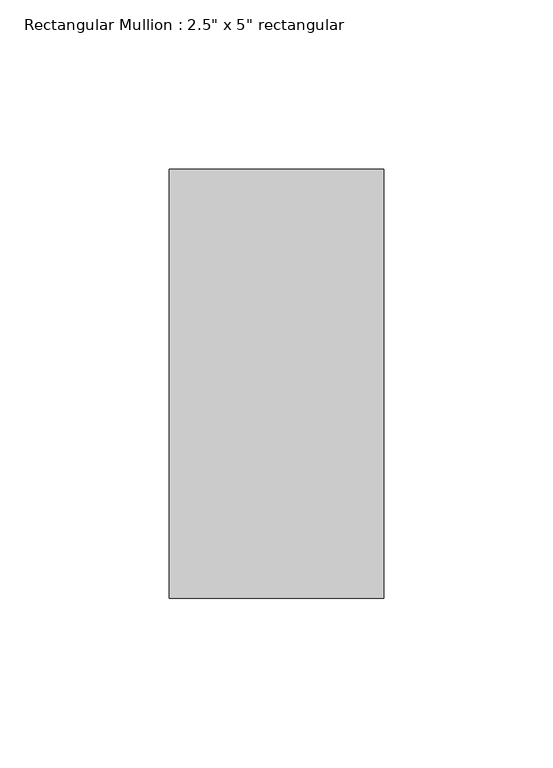
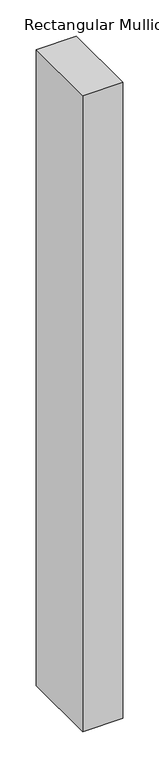
"""IFC4 building model written with IfcOpenShell, lengths in millimetres: member geometry."""

from ifc_helpers import new_model, si_unit, frame, origin, place, context, project, spatial, polyline, outline, extrude, source, transform, mapped, element, save


def member_2094b4cc(model_context):
    return source(origin(), model_context, "Body", "SweptSolid", [
        extrude(outline(polyline([(0.0, 63.5), (0.0, -63.5), (-63.5, -63.5), (-63.5, 63.5), (0.0, 63.5)])), frame((0.0, 0.0, -1067.0646279), z_axis=(0.0, 0.0, 1.0), x_axis=(1.0, 0.0, 0.0)), (0.0, 0.0, 1.0), 1067.0646279),
    ])


if __name__ == "__main__":
    model = new_model("IFC4")
    model_context = context("Model", 3, world=origin())
    ifc_project = project(units=[si_unit("LENGTHUNIT", "METRE", prefix="MILLI")], contexts=[model_context])
    site = spatial("IfcSite", under=ifc_project)
    building = spatial("IfcBuilding", under=site)
    placement = place(None, origin())
    member_shape = member_2094b4cc(model_context)
    element("IfcMember", 1, ObjectType="Rectangular Mullion : 2.5\" x 5\" rectangular", at=placement, inside=building, context=model_context, shape_type="MappedRepresentation", body=[
        mapped(member_shape, transform((0.0, 0.0, 0.0), x_axis=(1.0, 0.0, 0.0), y_axis=(0.0, 1.0, 0.0), z_axis=(0.0, 0.0, 1.0))),
    ])
    save(model, "model.ifc")

# Revit data of these elements
# Type "Rectangular Mullion : 2.5\" x 5\" rectangular"
#   built-in parameter 1007304 = 0.416667 (stored number, unit not read)
#   built-in parameter 1007301 = 0.104167 (stored number, unit not read)
#   built-in parameter 1007300 = 0.104167 (stored number, unit not read)
# Element 1 (IfcMember, "Rectangular Mullion : 2.5\" x 5\" rectangular")
#   Materials on its faces: "Aluminum"
# Materials
#   "Aluminum": class "Metal", colour RGB 247 247 247, transparency 0, Description = "Aluminum 6061", Cost = 0
